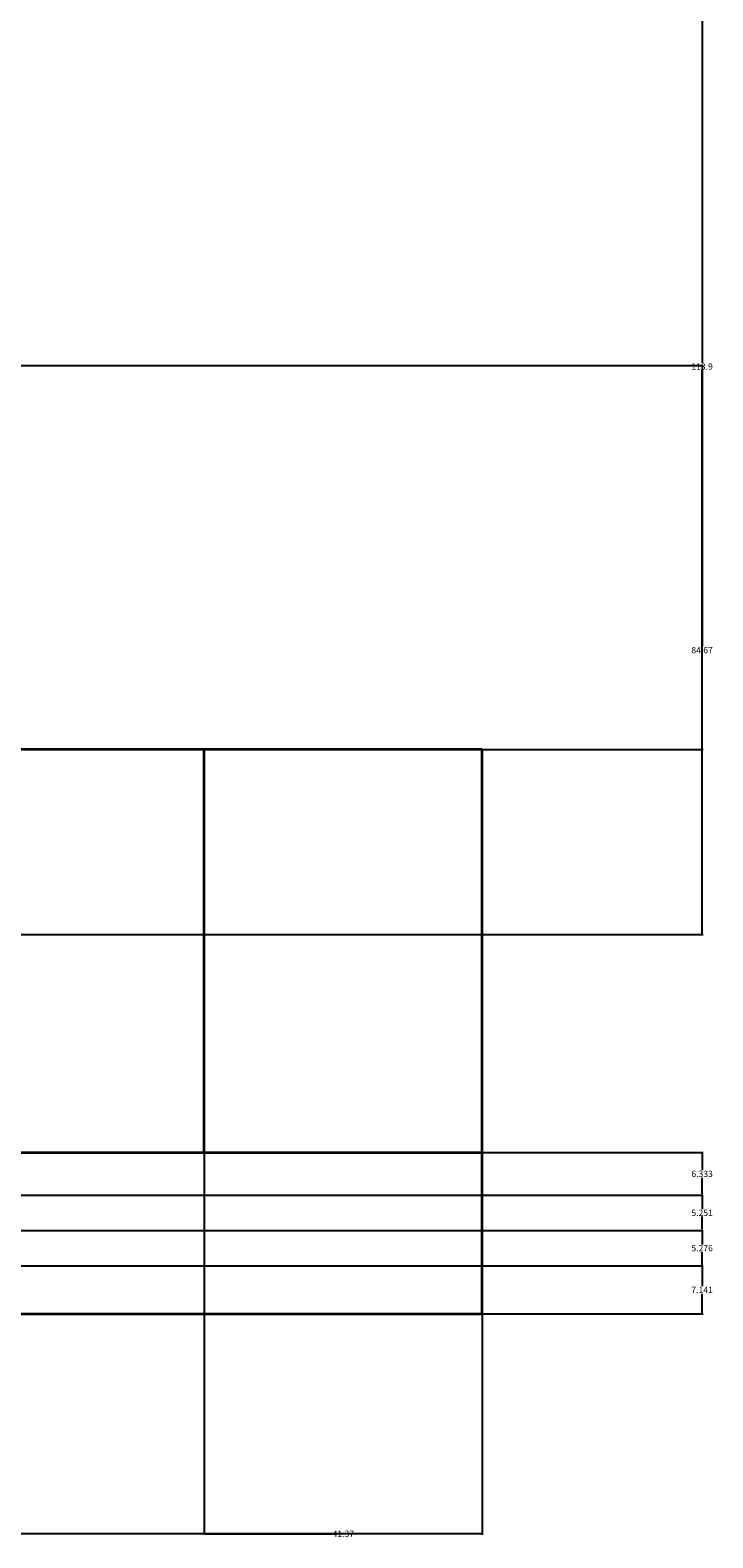
# Model space of a CAD drawing. Units: inches. Extents: x -5 to 714, y 84 to 644.
# Tile 17 of 20: x 613 to 714, y 84 to 308. Entities that reach past the tile are written whole.
import ezdxf

# ---------------------------------------------------------------- set-up
doc = ezdxf.new("R2010")
doc.units = ezdxf.units.IN
doc.header["$MEASUREMENT"] = 0
doc.layers.add('A-ANNO-DIMS', color=2, linetype='Continuous', lineweight=18)
doc.layers.add('A-ELEV', color=7, linetype='Continuous', lineweight=35)
doc.styles.get("Standard").update_dxf_attribs({"font": 'arial.ttf'})
doc.dimstyles.get("Standard").update_dxf_attribs({"dimtxt": 0.9375, "dimasz": 0.18, "dimexe": 0.18, "dimexo": 0.0625, "dimgap": 0.09, "dimtad": 0, "dimtih": 1, "dimtoh": 1, "dimdec": 4, "dimzin": 0, "dimdsep": 46, "dimlunit": 4, "dimtxsty": 'Standard', "dimcen": 0.09, "dimadec": 0, "dimazin": 0, "dimtfac": 1, "dimtdec": 4, "dimtofl": 0, "dimtmove": 0, "dimatfit": 3, "dimfxl": 1, "dimtolj": 1, "dimtzin": 0, "dimarcsym": 0})

# ---------------------------------------------------------------- blocks, each defined once
blk = doc.blocks.new('*D1')
at = {"layer": 'A-ANNO-DIMS', "color": 0, "lineweight": -2, "transparency": 16777216}
for p, q in [((30.14, 117.13), (30.14, 84.31)), ((679.78, 117.13), (679.78, 84.31)), ((30.32, 84.49), (353.29, 84.49)), ((679.6, 84.49), (356.64, 84.49))]:
    blk.add_line(p, q, dxfattribs=at)
at = {"layer": 'A-ANNO-DIMS', "color": 0, "transparency": 16777216}
for points in [[(30.32, 84.52), (30.32, 84.46), (30.14, 84.49)], [(679.6, 84.52), (679.6, 84.46), (679.78, 84.49)]]:
    blk.add_solid(points, dxfattribs=at)
at = {"layer": 'Defpoints', "color": 0, "transparency": 16777216}
for p in [(30.14, 117.19), (679.78, 117.19), (679.78, 84.49)]:
    blk.add_point(p, dxfattribs=at)
at = {"layer": 'A-ANNO-DIMS', "color": 0, "transparency": 16777216, "insert": (354.96, 84.49), "char_height": 0.938, "attachment_point": 5}
blk.add_mtext('\\A1;649.6', dxfattribs=at)
blk = doc.blocks.new('*D55')
at = {"layer": 'A-ANNO-DIMS', "color": 0, "lineweight": -2, "transparency": 16777216}
for p, q in [((593.49, 315.1), (712.66, 315.1)), ((712.48, 314.92), (712.48, 258.71)), ((712.48, 201.37), (712.48, 257.58)), ((593.49, 201.19), (712.66, 201.19))]:
    blk.add_line(p, q, dxfattribs=at)
at = {"layer": 'A-ANNO-DIMS', "color": 0, "transparency": 16777216}
for points in [[(712.45, 314.92), (712.51, 314.92), (712.48, 315.1)], [(712.45, 201.37), (712.51, 201.37), (712.48, 201.19)]]:
    blk.add_solid(points, dxfattribs=at)
at = {"layer": 'Defpoints', "color": 0, "transparency": 16777216}
for p in [(593.43, 315.1), (712.48, 315.1), (593.43, 201.19)]:
    blk.add_point(p, dxfattribs=at)
at = {"layer": 'A-ANNO-DIMS', "color": 0, "transparency": 16777216, "insert": (712.48, 258.14), "char_height": 0.938, "attachment_point": 5}
blk.add_mtext('\\A1;113.9', dxfattribs=at)
blk = doc.blocks.new('*D69')
at = {"layer": 'A-ANNO-DIMS', "color": 0, "lineweight": -2, "transparency": 16777216}
for p, q in [((403.5, 258.29), (712.66, 258.29)), ((712.48, 258.11), (712.48, 216.52)), ((712.48, 173.8), (712.48, 215.38)), ((403.5, 173.62), (712.66, 173.62))]:
    blk.add_line(p, q, dxfattribs=at)
at = {"layer": 'A-ANNO-DIMS', "color": 0, "transparency": 16777216}
for points in [[(712.45, 258.11), (712.51, 258.11), (712.48, 258.29)], [(712.45, 173.8), (712.51, 173.8), (712.48, 173.62)]]:
    blk.add_solid(points, dxfattribs=at)
at = {"layer": 'Defpoints', "color": 0, "transparency": 16777216}
for p in [(403.44, 258.29), (712.48, 258.29), (403.44, 173.62)]:
    blk.add_point(p, dxfattribs=at)
at = {"layer": 'A-ANNO-DIMS', "color": 0, "transparency": 16777216, "insert": (712.48, 215.95), "char_height": 0.938, "attachment_point": 5}
blk.add_mtext('\\A1;84.67', dxfattribs=at)
blk = doc.blocks.new('*D79')
at = {"layer": 'A-ANNO-DIMS', "color": 0, "lineweight": -2, "transparency": 16777216}
for p, q in [((543.72, 141.13), (543.72, 84.31)), ((638.41, 141.13), (638.41, 84.31)), ((543.9, 84.49), (589.76, 84.49)), ((638.23, 84.49), (592.37, 84.49))]:
    blk.add_line(p, q, dxfattribs=at)
at = {"layer": 'A-ANNO-DIMS', "color": 0, "transparency": 16777216}
for points in [[(543.9, 84.52), (543.9, 84.46), (543.72, 84.49)], [(638.23, 84.52), (638.23, 84.46), (638.41, 84.49)]]:
    blk.add_solid(points, dxfattribs=at)
at = {"layer": 'Defpoints', "color": 0, "transparency": 16777216}
for p in [(543.72, 141.19), (638.41, 141.19), (638.41, 84.49)]:
    blk.add_point(p, dxfattribs=at)
at = {"layer": 'A-ANNO-DIMS', "color": 0, "transparency": 16777216, "insert": (591.07, 84.49), "char_height": 0.938, "attachment_point": 5}
blk.add_mtext('\\A1;94.7', dxfattribs=at)
blk = doc.blocks.new('*D80')
at = {"layer": 'A-ANNO-DIMS', "color": 0, "lineweight": -2, "transparency": 16777216}
for p, q in [((638.41, 141.13), (638.41, 84.31)), ((679.78, 141.13), (679.78, 84.31)), ((638.59, 84.49), (657.41, 84.49)), ((679.6, 84.49), (660.79, 84.49))]:
    blk.add_line(p, q, dxfattribs=at)
at = {"layer": 'A-ANNO-DIMS', "color": 0, "transparency": 16777216}
for points in [[(638.59, 84.52), (638.59, 84.46), (638.41, 84.49)], [(679.6, 84.52), (679.6, 84.46), (679.78, 84.49)]]:
    blk.add_solid(points, dxfattribs=at)
at = {"layer": 'Defpoints', "color": 0, "transparency": 16777216}
for p in [(638.41, 141.19), (679.78, 141.19), (679.78, 84.49)]:
    blk.add_point(p, dxfattribs=at)
at = {"layer": 'A-ANNO-DIMS', "color": 0, "transparency": 16777216, "insert": (659.1, 84.49), "char_height": 0.938, "attachment_point": 5}
blk.add_mtext('\\A1;41.37', dxfattribs=at)
blk = doc.blocks.new('*D90')
at = {"layer": 'A-ANNO-DIMS', "color": 0, "lineweight": -2, "transparency": 16777216}
for p, q in [((543.78, 124.33), (712.66, 124.33)), ((712.48, 124.15), (712.48, 121.32)), ((712.48, 117.37), (712.48, 120.2)), ((543.78, 117.19), (712.66, 117.19))]:
    blk.add_line(p, q, dxfattribs=at)
at = {"layer": 'A-ANNO-DIMS', "color": 0, "transparency": 16777216}
for points in [[(712.45, 124.15), (712.51, 124.15), (712.48, 124.33)], [(712.45, 117.37), (712.51, 117.37), (712.48, 117.19)]]:
    blk.add_solid(points, dxfattribs=at)
at = {"layer": 'Defpoints', "color": 0, "transparency": 16777216}
for p in [(543.72, 124.33), (712.48, 124.33), (543.72, 117.19)]:
    blk.add_point(p, dxfattribs=at)
at = {"layer": 'A-ANNO-DIMS', "color": 0, "transparency": 16777216, "insert": (712.48, 120.76), "char_height": 0.938, "attachment_point": 5}
blk.add_mtext('\\A1;7.141', dxfattribs=at)
blk = doc.blocks.new('*D91')
at = {"layer": 'A-ANNO-DIMS', "color": 0, "lineweight": -2, "transparency": 16777216}
for p, q in [((543.78, 129.61), (712.66, 129.61)), ((712.48, 129.43), (712.48, 127.54)), ((712.48, 124.51), (712.48, 126.4)), ((543.78, 124.33), (712.66, 124.33))]:
    blk.add_line(p, q, dxfattribs=at)
at = {"layer": 'A-ANNO-DIMS', "color": 0, "transparency": 16777216}
for points in [[(712.45, 129.43), (712.51, 129.43), (712.48, 129.61)], [(712.45, 124.51), (712.51, 124.51), (712.48, 124.33)]]:
    blk.add_solid(points, dxfattribs=at)
at = {"layer": 'Defpoints', "color": 0, "transparency": 16777216}
for p in [(543.72, 129.61), (712.48, 129.61), (543.72, 124.33)]:
    blk.add_point(p, dxfattribs=at)
at = {"layer": 'A-ANNO-DIMS', "color": 0, "transparency": 16777216, "insert": (712.48, 126.97), "char_height": 0.938, "attachment_point": 5}
blk.add_mtext('\\A1;5.276', dxfattribs=at)
blk = doc.blocks.new('*D92')
at = {"layer": 'A-ANNO-DIMS', "color": 0, "lineweight": -2, "transparency": 16777216}
for p, q in [((543.78, 134.86), (712.66, 134.86)), ((712.48, 134.68), (712.48, 132.8)), ((712.48, 129.79), (712.48, 131.67)), ((543.78, 129.61), (712.66, 129.61))]:
    blk.add_line(p, q, dxfattribs=at)
at = {"layer": 'A-ANNO-DIMS', "color": 0, "transparency": 16777216}
for points in [[(712.45, 134.68), (712.51, 134.68), (712.48, 134.86)], [(712.45, 129.79), (712.51, 129.79), (712.48, 129.61)]]:
    blk.add_solid(points, dxfattribs=at)
at = {"layer": 'Defpoints', "color": 0, "transparency": 16777216}
for p in [(543.72, 134.86), (712.48, 134.86), (543.72, 129.61)]:
    blk.add_point(p, dxfattribs=at)
at = {"layer": 'A-ANNO-DIMS', "color": 0, "transparency": 16777216, "insert": (712.48, 132.23), "char_height": 0.938, "attachment_point": 5}
blk.add_mtext('\\A1;5.251', dxfattribs=at)
blk = doc.blocks.new('*D93')
at = {"layer": 'A-ANNO-DIMS', "color": 0, "lineweight": -2, "transparency": 16777216}
for p, q in [((543.78, 141.19), (712.66, 141.19)), ((712.48, 141.01), (712.48, 138.6)), ((712.48, 135.04), (712.48, 137.46)), ((543.78, 134.86), (712.66, 134.86))]:
    blk.add_line(p, q, dxfattribs=at)
at = {"layer": 'A-ANNO-DIMS', "color": 0, "transparency": 16777216}
for points in [[(712.45, 141.01), (712.51, 141.01), (712.48, 141.19)], [(712.45, 135.04), (712.51, 135.04), (712.48, 134.86)]]:
    blk.add_solid(points, dxfattribs=at)
at = {"layer": 'Defpoints', "color": 0, "transparency": 16777216}
for p in [(543.72, 141.19), (712.48, 141.19), (543.72, 134.86)]:
    blk.add_point(p, dxfattribs=at)
at = {"layer": 'A-ANNO-DIMS', "color": 0, "transparency": 16777216, "insert": (712.48, 138.03), "char_height": 0.938, "attachment_point": 5}
blk.add_mtext('\\A1;6.333', dxfattribs=at)

msp = doc.modelspace()

# ---------------------------------------------------------------- linework, layer by layer
at = {"layer": 'A-ELEV'}
for p, q in [((545.1065, 201.1928), (679.7826, 201.1928)), ((638.4139, 141.1928), (638.4139, 201.1928)), ((679.7826, 141.1928), (679.7826, 201.1928)), ((548.9353, 141.1928), (679.7826, 141.1928)), ((679.7826, 117.1928), (679.7826, 141.1928)), ((548.9353, 117.1928), (679.7826, 117.1928))]:
    msp.add_line(p, q, dxfattribs=at)

# ---------------------------------------------------------------- dimensions: what is measured, and where the dimension line sits
at = {"layer": 'A-ANNO-DIMS'}
for base, p1, p2, override, picture, middle in [((712.4826, 315.0968), (593.428, 201.1928), (593.428, 315.0968), {"dimdec": 1, "dimlfac": 1, "dimrnd": 0, "dimzin": 0, "dimdsep": 46, "dimlunit": 2}, '*D55', (712.4826, 258.1448)), ((712.4826, 258.2864), (403.4391, 173.6169), (403.4391, 258.2864), {"dimdec": 2, "dimlfac": 1, "dimrnd": 0, "dimzin": 0, "dimdsep": 46, "dimlunit": 2}, '*D69', (712.4826, 215.9517)), ((712.4826, 141.1928), (543.7164, 134.8602), (543.7164, 141.1928), {"dimdec": 3, "dimlfac": 1, "dimrnd": 0, "dimzin": 0, "dimdsep": 46, "dimlunit": 2}, '*D93', (712.4826, 138.0265)), ((712.4826, 134.8602), (543.7164, 129.6093), (543.7164, 134.8602), {"dimdec": 3, "dimlfac": 1, "dimrnd": 0, "dimzin": 0, "dimdsep": 46, "dimlunit": 2}, '*D92', (712.4826, 132.2347)), ((712.4826, 129.6093), (543.7164, 124.3337), (543.7164, 129.6093), {"dimdec": 3, "dimlfac": 1, "dimrnd": 0, "dimzin": 0, "dimdsep": 46, "dimlunit": 2}, '*D91', (712.4826, 126.9715)), ((712.4826, 124.3337), (543.7164, 117.1928), (543.7164, 124.3337), {"dimdec": 3, "dimlfac": 1, "dimrnd": 0, "dimzin": 0, "dimdsep": 46, "dimlunit": 2}, '*D90', (712.4826, 120.7633))]:
    dim = msp.add_linear_dim(base=base, p1=p1, p2=p2, angle=90, dimstyle='Standard', override=override, dxfattribs=at)
    dim.commit()
    dim.dimension.update_dxf_attribs({"geometry": picture, "text_midpoint": middle})
for base, p1, p2, override, picture, middle in [((638.4139, 84.4928), (543.7164, 141.1928), (638.4139, 141.1928), {"dimdec": 1, "dimlfac": 1, "dimrnd": 0, "dimzin": 0, "dimdsep": 46, "dimlunit": 2}, '*D79', (591.0652, 84.4928)), ((679.7826, 84.4928), (638.4139, 141.1928), (679.7826, 141.1928), {"dimdec": 2, "dimlfac": 1, "dimrnd": 0, "dimzin": 0, "dimdsep": 46, "dimlunit": 2}, '*D80', (659.0983, 84.4928)), ((679.7826, 84.4928), (30.1395, 117.1928), (679.7826, 117.1928), {"dimdec": 1, "dimlfac": 1, "dimrnd": 0, "dimzin": 0, "dimdsep": 46, "dimlunit": 2}, '*D1', (354.9611, 84.4928))]:
    dim = msp.add_linear_dim(base=base, p1=p1, p2=p2, dimstyle='Standard', override=override, dxfattribs=at)
    dim.commit()
    dim.dimension.update_dxf_attribs({"geometry": picture, "text_midpoint": middle})

doc.saveas('drawing.dxf')
